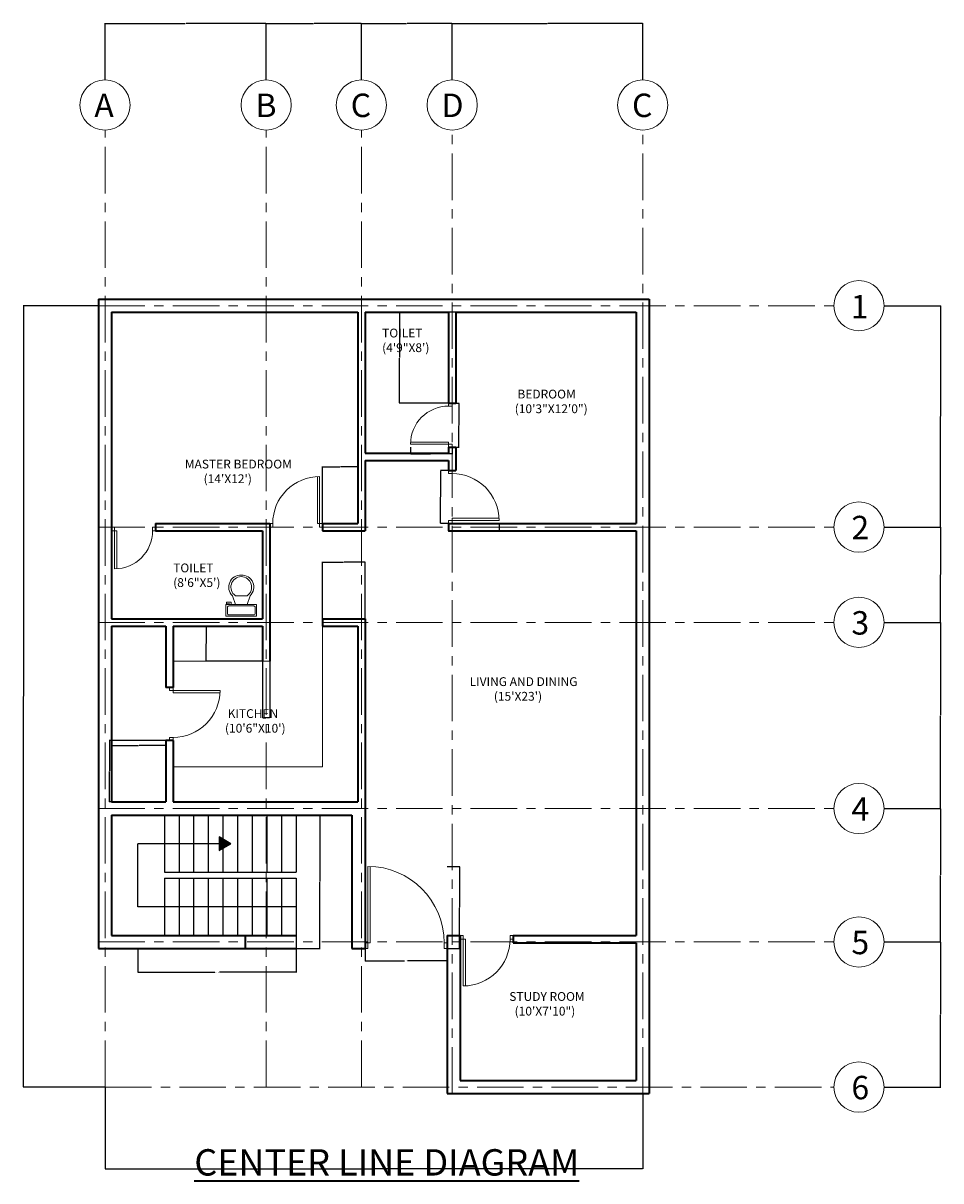
# Model space of a CAD drawing. Units: inches. Extents: x 2948 to 4025, y 2171 to 2966.
# Tile 6 of 6: x 3398 to 4025, y 2177 to 2966. Entities that reach past the tile are written whole.
import ezdxf

# ---------------------------------------------------------------- set-up
doc = ezdxf.new("R2010")
doc.units = ezdxf.units.IN
doc.linetypes.add('CENTER', pattern=[50.8, 31.75, -6.35, 6.35, -6.35])
for name, color, linetype, lineweight in [('A-ANNO-DIMS', 2, 'Continuous', 18), ('A-ANNO-TEXT', 7, 'Continuous', 35), ('A-AREA-IDEN', 7, 'Continuous', 18), ('A-DOOR', 3, 'Continuous', 18), ('A-FLOR-CASE', 8, 'Continuous', 18), ('A-FLOR-FIXT', 9, 'Continuous', 18), ('A-FLOR-STRS', 7, 'Continuous', 25), ('A-GRID', 1, 'CENTER', 13), ('A-GRID-IDEN', 7, 'Continuous', 18), ('A-WALL', 7, 'Continuous', 35)]:
    doc.layers.add(name, color=color, linetype=linetype, lineweight=lineweight)
doc.styles.get("Standard").update_dxf_attribs({"font": 'arial.ttf'})
doc.dimstyles.get("Standard").update_dxf_attribs({"dimtxt": 0.18, "dimasz": 0.18, "dimexe": 0.18, "dimexo": 0.0625, "dimgap": 0.09, "dimtad": 0, "dimtih": 1, "dimtoh": 1, "dimdec": 4, "dimzin": 0, "dimdsep": 46, "dimtxsty": 'Standard', "dimcen": 0.09, "dimadec": 0, "dimazin": 0, "dimtfac": 1, "dimtdec": 4, "dimtofl": 0, "dimtmove": 0, "dimatfit": 3, "dimfxl": 1, "dimtolj": 1, "dimtzin": 0, "dimarcsym": 0})

# ---------------------------------------------------------------- blocks, each defined once
blk = doc.blocks.new('*U8')
for p, q in [((9.5, -6), (9.5, -2)), ((-10, -8.5), (-8, -8.5)), ((-10, -9.5), (-10, -8.5)), ((-7, -9.5), (-10, -9.5)), ((-8, -8.5), (-8, -8)), ((-7, -8), (-7, -9.5)), ((-4, -8), (-6, -14)), ((4, -14), (-4, -14)), ((4, -8), (6, -14))]:
    blk.add_line(p, q)
blk.add_lwpolyline([(10.5, -8), (10.5, 0), (-10.5, 0), (-10.5, -8)], close=True)
for points in [[(-9.5, -2), (-9.5, -6)], [(8.5, -1), (-8.5, -1)], [(-8.5, -7), (8.5, -7)]]:
    blk.add_lwpolyline(points)
for centre, radius, start, end in [((-8.625, -1.875), 0.8839, 81.8699, 188.1301), ((-8.625, -6.125), 0.8839, 171.869898, 278.1301), ((8.625, -1.875), 0.8839, 351.8699, 98.1301), ((8.625, -6.125), 0.8839, 261.8699, 8.1301), ((-0.4772, -19.9188), 8.0953, 133.01722, 273.38), ((0.0374, -19.8731), 7.127, 124.50543, 269.7), ((-0.0373, -19.8731), 7.127, 270.3, 55.4946), ((0.4773, -19.9188), 8.0953, 266.62, 46.9828)]:
    blk.add_arc(centre, radius, start, end)
blk = doc.blocks.new('DOOR-SWING-32IN')
for p, q in [((2, 34.5), (0, 34.5)), ((0, 32), (2, 32)), ((2, 32), (2, 34.5)), ((2, 32), (2, 0)), ((2, 32), (3.5, 32)), ((3.5, 32), (3.5, 0.04)), ((34, 32), (34, 34.5)), ((34, 34.5), (36, 34.5)), ((36, 32), (34, 32))]:
    blk.add_line(p, q)
blk.add_arc((2, 32), 32, 270, 0)
blk = doc.blocks.new('DOOR-SWING-26IN')
for p, q in [((26, 30), (26, 28)), ((26, 28), (28.5, 28)), ((28.5, 28), (28.5, 30)), ((26, 2), (0, 2)), ((26, 3.5), (0.04, 3.5)), ((26, 3.5), (26, 2)), ((26, 0), (26, 2)), ((26, 2), (28.5, 2)), ((28.5, 2), (28.5, 0))]:
    blk.add_line(p, q)
blk.add_arc((26, 2), 26, 90, 180)
blk = doc.blocks.new('DOOR-ENTRY-52IN')
for p, q in [((2, 4), (2, 56)), ((3.5, 4), (3.5, 55.98)), ((2, 4), (0, 4)), ((0, 0), (2, 0)), ((2, 0), (2, 4)), ((2, 4), (3.5, 4)), ((54, 0), (54, 4)), ((54, 4), (56, 4)), ((56, 0), (54, 0))]:
    blk.add_line(p, q)
blk.add_arc((2, 4), 52, 0, 90)
blk = doc.blocks.new('STAIR-RETURN-FLIGHT')
h = blk.add_hatch(color=256)
h.dxf.hatch_style = 1
h.paths.add_polyline_path([(63.35, 71.5), (55.35, 76.12), (55.35, 66.88)])
for p, q in [((18.02, 91), (18.02, 52)), ((28.02, 91), (28.02, 52)), ((38.02, 91), (38.02, 52)), ((48.02, 91), (48.02, 52)), ((58.02, 91), (58.02, 74.58)), ((68.02, 91), (68.02, 52)), ((78.02, 91), (78.02, 52)), ((88.02, 91), (88.02, 52)), ((98.02, 91), (98.02, 52)), ((108.02, 91), (108.02, 52)), ((0, 28.5), (0, 71.5)), ((55.35, 71.5), (0, 71.5)), ((58.02, 68.42), (58.02, 52)), ((18.02, 52), (108.02, 52)), ((18.02, 48), (108.02, 48)), ((18.02, 48), (18.02, 9)), ((28.02, 48), (28.02, 9)), ((38.02, 48), (38.02, 9)), ((48.02, 48), (48.02, 9)), ((58.02, 48), (58.02, 9)), ((68.02, 48), (68.02, 9)), ((78.02, 48), (78.02, 9)), ((88.02, 48), (88.02, 9)), ((98.02, 48), (98.02, 9)), ((108.02, 48), (108.02, 0)), ((108.02, 28.5), (0, 28.5))]:
    blk.add_line(p, q)
blk.add_lwpolyline([(63.35, 71.5), (55.35, 76.12), (55.35, 66.88)], close=True)
blk = doc.blocks.new('*D15')
at = {"layer": 'A-ANNO-DIMS', "color": 0, "lineweight": -2, "transparency": 16777216}
for p, q in [((3688.78, 2660.99), (3683.26, 2660.99)), ((3683.44, 2660.81), (3683.44, 2643.17)), ((3683.44, 2625.17), (3683.44, 2642.8)), ((3688.78, 2624.99), (3683.26, 2624.99))]:
    blk.add_line(p, q, dxfattribs=at)
at = {"layer": 'A-ANNO-DIMS', "color": 0, "transparency": 16777216}
for points in [[(3683.41, 2660.81), (3683.47, 2660.81), (3683.44, 2660.99)], [(3683.41, 2625.17), (3683.47, 2625.17), (3683.44, 2624.99)]]:
    blk.add_solid(points, dxfattribs=at)
at = {"layer": 'Defpoints', "color": 0, "transparency": 16777216}
for p in [(3683.44, 2660.99), (3688.84, 2660.99), (3688.84, 2624.99)]:
    blk.add_point(p, dxfattribs=at)
at = {"layer": 'A-ANNO-DIMS', "color": 0, "transparency": 16777216, "insert": (3683.44, 2642.99), "char_height": 0.18, "attachment_point": 5}
blk.add_mtext('\\A1;ROOM DOOR 36 TYP.', dxfattribs=at)
blk = doc.blocks.new('*D16')
at = {"layer": 'A-ANNO-DIMS', "color": 0, "lineweight": -2, "transparency": 16777216}
for p, q in [((3688.84, 2624.92), (3688.84, 2619.41)), ((3723.34, 2624.92), (3723.34, 2619.41)), ((3689.02, 2619.59), (3705.56, 2619.59)), ((3723.16, 2619.59), (3706.62, 2619.59))]:
    blk.add_line(p, q, dxfattribs=at)
at = {"layer": 'A-ANNO-DIMS', "color": 0, "transparency": 16777216}
for points in [[(3689.02, 2619.62), (3689.02, 2619.56), (3688.84, 2619.59)], [(3723.16, 2619.62), (3723.16, 2619.56), (3723.34, 2619.59)]]:
    blk.add_solid(points, dxfattribs=at)
at = {"layer": 'Defpoints', "color": 0, "transparency": 16777216}
for p in [(3688.84, 2624.99), (3723.34, 2624.99), (3688.84, 2619.59)]:
    blk.add_point(p, dxfattribs=at)
at = {"layer": 'A-ANNO-DIMS', "color": 0, "transparency": 16777216, "insert": (3706.09, 2619.59), "char_height": 0.18, "attachment_point": 5}
blk.add_mtext('\\A1;35 TYP.', dxfattribs=at)
blk = doc.blocks.new('*D17')
at = {"layer": 'A-ANNO-DIMS', "color": 0, "lineweight": -2, "transparency": 16777216}
for p, q in [((3691.4, 2706.99), (3696.02, 2706.99)), ((3695.84, 2706.81), (3695.84, 2692.17)), ((3695.84, 2677.17), (3695.84, 2691.8)), ((3691.4, 2676.99), (3696.02, 2676.99))]:
    blk.add_line(p, q, dxfattribs=at)
at = {"layer": 'A-ANNO-DIMS', "color": 0, "transparency": 16777216}
for points in [[(3695.81, 2706.81), (3695.87, 2706.81), (3695.84, 2706.99)], [(3695.81, 2677.17), (3695.87, 2677.17), (3695.84, 2676.99)]]:
    blk.add_solid(points, dxfattribs=at)
at = {"layer": 'Defpoints', "color": 0, "transparency": 16777216}
for p in [(3691.34, 2706.99), (3695.84, 2706.99), (3691.34, 2676.99)]:
    blk.add_point(p, dxfattribs=at)
at = {"layer": 'A-ANNO-DIMS', "color": 0, "transparency": 16777216, "insert": (3695.84, 2691.99), "char_height": 0.18, "attachment_point": 5}
blk.add_mtext('\\A1;WC DOOR 30 TYP.', dxfattribs=at)
blk = doc.blocks.new('*D18')
at = {"layer": 'A-ANNO-DIMS', "color": 0, "lineweight": -2, "transparency": 16777216}
for p, q in [((3662.84, 2676.92), (3662.84, 2672.31)), ((3663.02, 2672.49), (3676.56, 2672.49)), ((3691.16, 2672.49), (3677.62, 2672.49)), ((3691.34, 2676.92), (3691.34, 2672.31))]:
    blk.add_line(p, q, dxfattribs=at)
at = {"layer": 'A-ANNO-DIMS', "color": 0, "transparency": 16777216}
for points in [[(3663.02, 2672.52), (3663.02, 2672.46), (3662.84, 2672.49)], [(3691.16, 2672.52), (3691.16, 2672.46), (3691.34, 2672.49)]]:
    blk.add_solid(points, dxfattribs=at)
at = {"layer": 'Defpoints', "color": 0, "transparency": 16777216}
for p in [(3662.84, 2676.99), (3691.34, 2676.99), (3691.34, 2672.49)]:
    blk.add_point(p, dxfattribs=at)
at = {"layer": 'A-ANNO-DIMS', "color": 0, "transparency": 16777216, "insert": (3677.09, 2672.49), "char_height": 0.18, "attachment_point": 5}
blk.add_mtext('\\A1;29 TYP.', dxfattribs=at)
blk = doc.blocks.new('*D19')
at = {"layer": 'A-ANNO-DIMS', "color": 0, "lineweight": -2, "transparency": 16777216}
for p, q in [((3631.84, 2334.92), (3631.84, 2326.41)), ((3687.84, 2334.92), (3687.84, 2326.41)), ((3632.02, 2326.59), (3658.85, 2326.59)), ((3687.66, 2326.59), (3660.82, 2326.59))]:
    blk.add_line(p, q, dxfattribs=at)
at = {"layer": 'A-ANNO-DIMS', "color": 0, "transparency": 16777216}
for points in [[(3632.02, 2326.62), (3632.02, 2326.56), (3631.84, 2326.59)], [(3687.66, 2326.62), (3687.66, 2326.56), (3687.84, 2326.59)]]:
    blk.add_solid(points, dxfattribs=at)
at = {"layer": 'Defpoints', "color": 0, "transparency": 16777216}
for p in [(3631.84, 2334.99), (3687.84, 2334.99), (3687.84, 2326.59)]:
    blk.add_point(p, dxfattribs=at)
at = {"layer": 'A-ANNO-DIMS', "color": 0, "transparency": 16777216, "insert": (3659.84, 2326.59), "char_height": 0.18, "attachment_point": 5}
blk.add_mtext('\\A1;ENTRY 56 TYP.', dxfattribs=at)
blk = doc.blocks.new('*D20')
at = {"layer": 'A-ANNO-DIMS', "color": 0, "lineweight": -2, "transparency": 16777216}
for p, q in [((3687.9, 2390.99), (3696.42, 2390.99)), ((3696.24, 2390.81), (3696.24, 2363.17)), ((3696.24, 2335.17), (3696.24, 2362.8)), ((3687.9, 2334.99), (3696.42, 2334.99))]:
    blk.add_line(p, q, dxfattribs=at)
at = {"layer": 'A-ANNO-DIMS', "color": 0, "transparency": 16777216}
for points in [[(3696.21, 2390.81), (3696.27, 2390.81), (3696.24, 2390.99)], [(3696.21, 2335.17), (3696.27, 2335.17), (3696.24, 2334.99)]]:
    blk.add_solid(points, dxfattribs=at)
at = {"layer": 'Defpoints', "color": 0, "transparency": 16777216}
for p in [(3687.84, 2390.99), (3696.24, 2390.99), (3687.84, 2334.99)]:
    blk.add_point(p, dxfattribs=at)
at = {"layer": 'A-ANNO-DIMS', "color": 0, "transparency": 16777216, "insert": (3696.24, 2362.99), "char_height": 0.18, "attachment_point": 5}
blk.add_mtext('\\A1;56 TYP.', dxfattribs=at)
blk = doc.blocks.new('*D25')
at = {"layer": 'A-ANNO-DIMS', "color": 0, "lineweight": -2, "transparency": 16777216}
for p, q in [((3476.82, 2334.92), (3476.82, 2318.6)), ((3584.84, 2334.92), (3584.84, 2318.6)), ((3477, 2318.78), (3529.27, 2318.78)), ((3584.66, 2318.78), (3532.39, 2318.78))]:
    blk.add_line(p, q, dxfattribs=at)
at = {"layer": 'A-ANNO-DIMS', "color": 0, "transparency": 16777216}
for points in [[(3477, 2318.81), (3477, 2318.75), (3476.82, 2318.78)], [(3584.66, 2318.81), (3584.66, 2318.75), (3584.84, 2318.78)]]:
    blk.add_solid(points, dxfattribs=at)
at = {"layer": 'Defpoints', "color": 0, "transparency": 16777216}
for p in [(3476.82, 2334.99), (3584.84, 2334.99), (3584.84, 2318.78)]:
    blk.add_point(p, dxfattribs=at)
at = {"layer": 'A-ANNO-DIMS', "color": 0, "transparency": 16777216, "insert": (3530.83, 2318.78), "char_height": 0.18, "attachment_point": 5}
blk.add_mtext('\\A1;RETURN STAIR 108 TYP.', dxfattribs=at)
blk = doc.blocks.new('*D26')
at = {"layer": 'A-ANNO-DIMS', "color": 0, "lineweight": -2, "transparency": 16777216}
for p, q in [((3584.9, 2425.99), (3601.22, 2425.99)), ((3601.04, 2425.81), (3601.04, 2380.67)), ((3601.04, 2335.17), (3601.04, 2380.3)), ((3584.9, 2334.99), (3601.22, 2334.99))]:
    blk.add_line(p, q, dxfattribs=at)
at = {"layer": 'A-ANNO-DIMS', "color": 0, "transparency": 16777216}
for points in [[(3601.01, 2425.81), (3601.07, 2425.81), (3601.04, 2425.99)], [(3601.01, 2335.17), (3601.07, 2335.17), (3601.04, 2334.99)]]:
    blk.add_solid(points, dxfattribs=at)
at = {"layer": 'Defpoints', "color": 0, "transparency": 16777216}
for p in [(3584.84, 2425.99), (3601.04, 2425.99), (3584.84, 2334.99)]:
    blk.add_point(p, dxfattribs=at)
at = {"layer": 'A-ANNO-DIMS', "color": 0, "transparency": 16777216, "insert": (3601.04, 2380.49), "char_height": 0.18, "attachment_point": 5}
blk.add_mtext('\\A1;91 TYP.', dxfattribs=at)
blk = doc.blocks.new('*D49')
at = {"layer": 'A-ANNO-DIMS', "color": 0, "lineweight": -2, "transparency": 16777216}
for p, q in [((3454.34, 2927.56), (3454.34, 2966.23)), ((3454.52, 2966.05), (3509.06, 2966.05)), ((3564.16, 2966.05), (3509.62, 2966.05)), ((3564.34, 2927.56), (3564.34, 2966.23))]:
    blk.add_line(p, q, dxfattribs=at)
at = {"layer": 'A-ANNO-DIMS', "color": 0, "transparency": 16777216}
for points in [[(3454.52, 2966.08), (3454.52, 2966.02), (3454.34, 2966.05)], [(3564.16, 2966.08), (3564.16, 2966.02), (3564.34, 2966.05)]]:
    blk.add_solid(points, dxfattribs=at)
at = {"layer": 'Defpoints', "color": 0, "transparency": 16777216}
for p in [(3564.34, 2966.05), (3454.34, 2927.5), (3564.34, 2927.5)]:
    blk.add_point(p, dxfattribs=at)
at = {"layer": 'A-ANNO-DIMS', "color": 0, "transparency": 16777216, "insert": (3509.34, 2966.05), "char_height": 0.18, "attachment_point": 5}
blk.add_mtext('\\A1;110', dxfattribs=at)
blk = doc.blocks.new('*D50')
at = {"layer": 'A-ANNO-DIMS', "color": 0, "lineweight": -2, "transparency": 16777216}
for p, q in [((3564.34, 2927.56), (3564.34, 2966.23)), ((3564.52, 2966.05), (3596.62, 2966.05)), ((3629.16, 2966.05), (3597.06, 2966.05)), ((3629.34, 2927.56), (3629.34, 2966.23))]:
    blk.add_line(p, q, dxfattribs=at)
at = {"layer": 'A-ANNO-DIMS', "color": 0, "transparency": 16777216}
for points in [[(3564.52, 2966.08), (3564.52, 2966.02), (3564.34, 2966.05)], [(3629.16, 2966.08), (3629.16, 2966.02), (3629.34, 2966.05)]]:
    blk.add_solid(points, dxfattribs=at)
at = {"layer": 'Defpoints', "color": 0, "transparency": 16777216}
for p in [(3629.34, 2966.05), (3564.34, 2927.5), (3629.34, 2927.5)]:
    blk.add_point(p, dxfattribs=at)
at = {"layer": 'A-ANNO-DIMS', "color": 0, "transparency": 16777216, "insert": (3596.84, 2966.05), "char_height": 0.18, "attachment_point": 5}
blk.add_mtext('\\A1;65', dxfattribs=at)
blk = doc.blocks.new('*D51')
at = {"layer": 'A-ANNO-DIMS', "color": 0, "lineweight": -2, "transparency": 16777216}
for p, q in [((3629.34, 2927.56), (3629.34, 2966.23)), ((3629.52, 2966.05), (3660.12, 2966.05)), ((3691.16, 2966.05), (3660.56, 2966.05)), ((3691.34, 2927.56), (3691.34, 2966.23))]:
    blk.add_line(p, q, dxfattribs=at)
at = {"layer": 'A-ANNO-DIMS', "color": 0, "transparency": 16777216}
for points in [[(3629.52, 2966.08), (3629.52, 2966.02), (3629.34, 2966.05)], [(3691.16, 2966.08), (3691.16, 2966.02), (3691.34, 2966.05)]]:
    blk.add_solid(points, dxfattribs=at)
at = {"layer": 'Defpoints', "color": 0, "transparency": 16777216}
for p in [(3691.34, 2966.05), (3629.34, 2927.5), (3691.34, 2927.5)]:
    blk.add_point(p, dxfattribs=at)
at = {"layer": 'A-ANNO-DIMS', "color": 0, "transparency": 16777216, "insert": (3660.34, 2966.05), "char_height": 0.18, "attachment_point": 5}
blk.add_mtext('\\A1;62', dxfattribs=at)
blk = doc.blocks.new('*D52')
at = {"layer": 'A-ANNO-DIMS', "color": 0, "lineweight": -2, "transparency": 16777216}
for p, q in [((3691.34, 2927.56), (3691.34, 2966.23)), ((3691.52, 2966.05), (3756.06, 2966.05)), ((3821.16, 2966.05), (3756.62, 2966.05)), ((3821.34, 2927.56), (3821.34, 2966.23))]:
    blk.add_line(p, q, dxfattribs=at)
at = {"layer": 'A-ANNO-DIMS', "color": 0, "transparency": 16777216}
for points in [[(3691.52, 2966.08), (3691.52, 2966.02), (3691.34, 2966.05)], [(3821.16, 2966.08), (3821.16, 2966.02), (3821.34, 2966.05)]]:
    blk.add_solid(points, dxfattribs=at)
at = {"layer": 'Defpoints', "color": 0, "transparency": 16777216}
for p in [(3821.34, 2966.05), (3691.34, 2927.5), (3821.34, 2927.5)]:
    blk.add_point(p, dxfattribs=at)
at = {"layer": 'A-ANNO-DIMS', "color": 0, "transparency": 16777216, "insert": (3756.34, 2966.05), "char_height": 0.18, "attachment_point": 5}
blk.add_mtext('\\A1;130', dxfattribs=at)
blk = doc.blocks.new('*D53')
at = {"layer": 'A-ANNO-DIMS', "color": 0, "lineweight": -2, "transparency": 16777216}
for p, q in [((3454.34, 2240.42), (3454.34, 2184.63)), ((3821.34, 2235.92), (3821.34, 2184.63)), ((3454.52, 2184.81), (3637.55, 2184.81)), ((3821.16, 2184.81), (3638.13, 2184.81))]:
    blk.add_line(p, q, dxfattribs=at)
at = {"layer": 'A-ANNO-DIMS', "color": 0, "transparency": 16777216}
for points in [[(3454.52, 2184.84), (3454.52, 2184.78), (3454.34, 2184.81)], [(3821.16, 2184.84), (3821.16, 2184.78), (3821.34, 2184.81)]]:
    blk.add_solid(points, dxfattribs=at)
at = {"layer": 'Defpoints', "color": 0, "transparency": 16777216}
for p in [(3454.34, 2240.49), (3821.34, 2235.99), (3821.34, 2184.81)]:
    blk.add_point(p, dxfattribs=at)
at = {"layer": 'A-ANNO-DIMS', "color": 0, "transparency": 16777216, "insert": (3637.84, 2184.81), "char_height": 0.18, "attachment_point": 5}
blk.add_mtext('\\A1;367', dxfattribs=at)
blk = doc.blocks.new('*D54')
at = {"layer": 'A-ANNO-DIMS', "color": 0, "lineweight": -2, "transparency": 16777216}
for p, q in [((3986.17, 2773.49), (4024.84, 2773.49)), ((4024.66, 2773.31), (4024.66, 2698.17)), ((4024.66, 2622.67), (4024.66, 2697.8)), ((3986.17, 2622.49), (4024.84, 2622.49))]:
    blk.add_line(p, q, dxfattribs=at)
at = {"layer": 'A-ANNO-DIMS', "color": 0, "transparency": 16777216}
for points in [[(4024.63, 2773.31), (4024.69, 2773.31), (4024.66, 2773.49)], [(4024.63, 2622.67), (4024.69, 2622.67), (4024.66, 2622.49)]]:
    blk.add_solid(points, dxfattribs=at)
at = {"layer": 'Defpoints', "color": 0, "transparency": 16777216}
for p in [(3986.11, 2773.49), (4024.66, 2773.49), (3986.11, 2622.49)]:
    blk.add_point(p, dxfattribs=at)
at = {"layer": 'A-ANNO-DIMS', "color": 0, "transparency": 16777216, "insert": (4024.66, 2697.99), "char_height": 0.18, "attachment_point": 5}
blk.add_mtext('\\A1;151', dxfattribs=at)
blk = doc.blocks.new('*D55')
at = {"layer": 'A-ANNO-DIMS', "color": 0, "lineweight": -2, "transparency": 16777216}
for p, q in [((3986.17, 2622.49), (4024.84, 2622.49)), ((4024.66, 2622.31), (4024.66, 2590.17)), ((4024.66, 2557.67), (4024.66, 2589.8)), ((3986.17, 2557.49), (4024.84, 2557.49))]:
    blk.add_line(p, q, dxfattribs=at)
at = {"layer": 'A-ANNO-DIMS', "color": 0, "transparency": 16777216}
for points in [[(4024.63, 2622.31), (4024.69, 2622.31), (4024.66, 2622.49)], [(4024.63, 2557.67), (4024.69, 2557.67), (4024.66, 2557.49)]]:
    blk.add_solid(points, dxfattribs=at)
at = {"layer": 'Defpoints', "color": 0, "transparency": 16777216}
for p in [(3986.11, 2622.49), (4024.66, 2622.49), (3986.11, 2557.49)]:
    blk.add_point(p, dxfattribs=at)
at = {"layer": 'A-ANNO-DIMS', "color": 0, "transparency": 16777216, "insert": (4024.66, 2589.99), "char_height": 0.18, "attachment_point": 5}
blk.add_mtext('\\A1;65', dxfattribs=at)
blk = doc.blocks.new('*D56')
at = {"layer": 'A-ANNO-DIMS', "color": 0, "lineweight": -2, "transparency": 16777216}
for p, q in [((3986.17, 2557.49), (4024.84, 2557.49)), ((4024.66, 2557.31), (4024.66, 2494.17)), ((4024.66, 2430.67), (4024.66, 2493.81)), ((3986.17, 2430.49), (4024.84, 2430.49))]:
    blk.add_line(p, q, dxfattribs=at)
at = {"layer": 'A-ANNO-DIMS', "color": 0, "transparency": 16777216}
for points in [[(4024.63, 2557.31), (4024.69, 2557.31), (4024.66, 2557.49)], [(4024.63, 2430.67), (4024.69, 2430.67), (4024.66, 2430.49)]]:
    blk.add_solid(points, dxfattribs=at)
at = {"layer": 'Defpoints', "color": 0, "transparency": 16777216}
for p in [(3986.11, 2557.49), (4024.66, 2557.49), (3986.11, 2430.49)]:
    blk.add_point(p, dxfattribs=at)
at = {"layer": 'A-ANNO-DIMS', "color": 0, "transparency": 16777216, "insert": (4024.66, 2493.99), "char_height": 0.18, "attachment_point": 5}
blk.add_mtext('\\A1;127', dxfattribs=at)
blk = doc.blocks.new('*D57')
at = {"layer": 'A-ANNO-DIMS', "color": 0, "lineweight": -2, "transparency": 16777216}
for p, q in [((3986.17, 2430.49), (4024.84, 2430.49)), ((4024.66, 2430.31), (4024.66, 2385.17)), ((4024.66, 2339.67), (4024.66, 2384.8)), ((3986.17, 2339.49), (4024.84, 2339.49))]:
    blk.add_line(p, q, dxfattribs=at)
at = {"layer": 'A-ANNO-DIMS', "color": 0, "transparency": 16777216}
for points in [[(4024.63, 2430.31), (4024.69, 2430.31), (4024.66, 2430.49)], [(4024.63, 2339.67), (4024.69, 2339.67), (4024.66, 2339.49)]]:
    blk.add_solid(points, dxfattribs=at)
at = {"layer": 'Defpoints', "color": 0, "transparency": 16777216}
for p in [(3986.11, 2430.49), (4024.66, 2430.49), (3986.11, 2339.49)]:
    blk.add_point(p, dxfattribs=at)
at = {"layer": 'A-ANNO-DIMS', "color": 0, "transparency": 16777216, "insert": (4024.66, 2384.99), "char_height": 0.18, "attachment_point": 5}
blk.add_mtext('\\A1;91', dxfattribs=at)
blk = doc.blocks.new('*D58')
at = {"layer": 'A-ANNO-DIMS', "color": 0, "lineweight": -2, "transparency": 16777216}
for p, q in [((3986.17, 2339.49), (4024.84, 2339.49)), ((4024.66, 2339.31), (4024.66, 2290.17)), ((4024.66, 2240.67), (4024.66, 2289.8)), ((3986.17, 2240.49), (4024.84, 2240.49))]:
    blk.add_line(p, q, dxfattribs=at)
at = {"layer": 'A-ANNO-DIMS', "color": 0, "transparency": 16777216}
for points in [[(4024.63, 2339.31), (4024.69, 2339.31), (4024.66, 2339.49)], [(4024.63, 2240.67), (4024.69, 2240.67), (4024.66, 2240.49)]]:
    blk.add_solid(points, dxfattribs=at)
at = {"layer": 'Defpoints', "color": 0, "transparency": 16777216}
for p in [(3986.11, 2339.49), (4024.66, 2339.49), (3986.11, 2240.49)]:
    blk.add_point(p, dxfattribs=at)
at = {"layer": 'A-ANNO-DIMS', "color": 0, "transparency": 16777216, "insert": (4024.66, 2289.99), "char_height": 0.18, "attachment_point": 5}
blk.add_mtext('\\A1;99', dxfattribs=at)
blk = doc.blocks.new('*D59')
at = {"layer": 'A-ANNO-DIMS', "color": 0, "lineweight": -2, "transparency": 16777216}
for p, q in [((3449.78, 2773.49), (3398.48, 2773.49)), ((3398.66, 2773.31), (3398.66, 2507.17)), ((3398.66, 2240.67), (3398.66, 2506.8)), ((3454.28, 2240.49), (3398.48, 2240.49))]:
    blk.add_line(p, q, dxfattribs=at)
at = {"layer": 'A-ANNO-DIMS', "color": 0, "transparency": 16777216}
for points in [[(3398.63, 2773.31), (3398.69, 2773.31), (3398.66, 2773.49)], [(3398.63, 2240.67), (3398.69, 2240.67), (3398.66, 2240.49)]]:
    blk.add_solid(points, dxfattribs=at)
at = {"layer": 'Defpoints', "color": 0, "transparency": 16777216}
for p in [(3398.66, 2773.49), (3449.84, 2773.49), (3454.34, 2240.49)]:
    blk.add_point(p, dxfattribs=at)
at = {"layer": 'A-ANNO-DIMS', "color": 0, "transparency": 16777216, "insert": (3398.66, 2506.99), "char_height": 0.18, "attachment_point": 5}
blk.add_mtext('\\A1;533', dxfattribs=at)
blk = doc.blocks.new('*D60')
at = {"layer": 'A-ANNO-DIMS', "color": 0, "lineweight": -2, "transparency": 16777216}
for p, q in [((3458.84, 2435.05), (3458.84, 2473.72)), ((3459.02, 2473.54), (3477.12, 2473.54)), ((3495.66, 2473.54), (3477.56, 2473.54)), ((3495.84, 2435.05), (3495.84, 2473.72))]:
    blk.add_line(p, q, dxfattribs=at)
at = {"layer": 'A-ANNO-DIMS', "color": 0, "transparency": 16777216}
for points in [[(3459.02, 2473.57), (3459.02, 2473.51), (3458.84, 2473.54)], [(3495.66, 2473.57), (3495.66, 2473.51), (3495.84, 2473.54)]]:
    blk.add_solid(points, dxfattribs=at)
at = {"layer": 'Defpoints', "color": 0, "transparency": 16777216}
for p in [(3495.84, 2473.54), (3458.84, 2434.99), (3495.84, 2434.99)]:
    blk.add_point(p, dxfattribs=at)
at = {"layer": 'A-ANNO-DIMS', "color": 0, "transparency": 16777216, "insert": (3477.34, 2473.54), "char_height": 0.18, "attachment_point": 5}
blk.add_mtext('\\A1;37', dxfattribs=at)
blk = doc.blocks.new('*D61')
at = {"layer": 'A-ANNO-DIMS', "color": 0, "lineweight": -2, "transparency": 16777216}
for p, q in [((3495.78, 2476.99), (3457.11, 2476.99)), ((3457.29, 2476.81), (3457.29, 2456.17)), ((3457.29, 2435.17), (3457.29, 2455.81)), ((3495.78, 2434.99), (3457.11, 2434.99))]:
    blk.add_line(p, q, dxfattribs=at)
at = {"layer": 'A-ANNO-DIMS', "color": 0, "transparency": 16777216}
for points in [[(3457.26, 2476.81), (3457.32, 2476.81), (3457.29, 2476.99)], [(3457.26, 2435.17), (3457.32, 2435.17), (3457.29, 2434.99)]]:
    blk.add_solid(points, dxfattribs=at)
at = {"layer": 'Defpoints', "color": 0, "transparency": 16777216}
for p in [(3457.29, 2476.99), (3495.84, 2476.99), (3495.84, 2434.99)]:
    blk.add_point(p, dxfattribs=at)
at = {"layer": 'A-ANNO-DIMS', "color": 0, "transparency": 16777216, "insert": (3457.29, 2455.99), "char_height": 0.18, "attachment_point": 5}
blk.add_mtext('\\A1;42', dxfattribs=at)
blk = doc.blocks.new('*D62')
at = {"layer": 'A-ANNO-DIMS', "color": 0, "lineweight": -2, "transparency": 16777216}
for p, q in [((3561.78, 2554.99), (3523.11, 2554.99)), ((3523.29, 2554.81), (3523.29, 2543.17)), ((3523.29, 2531.17), (3523.29, 2542.81)), ((3561.78, 2530.99), (3523.11, 2530.99))]:
    blk.add_line(p, q, dxfattribs=at)
at = {"layer": 'A-ANNO-DIMS', "color": 0, "transparency": 16777216}
for points in [[(3523.26, 2554.81), (3523.32, 2554.81), (3523.29, 2554.99)], [(3523.26, 2531.17), (3523.32, 2531.17), (3523.29, 2530.99)]]:
    blk.add_solid(points, dxfattribs=at)
at = {"layer": 'Defpoints', "color": 0, "transparency": 16777216}
for p in [(3523.29, 2554.99), (3561.84, 2554.99), (3561.84, 2530.99)]:
    blk.add_point(p, dxfattribs=at)
at = {"layer": 'A-ANNO-DIMS', "color": 0, "transparency": 16777216, "insert": (3523.29, 2542.99), "char_height": 0.18, "attachment_point": 5}
blk.add_mtext('\\A1;24', dxfattribs=at)
blk = doc.blocks.new('*D63')
at = {"layer": 'A-ANNO-DIMS', "color": 0, "lineweight": -2, "transparency": 16777216}
for p, q in [((3602.84, 2560.05), (3602.84, 2598.72)), ((3603.02, 2598.54), (3617.12, 2598.54)), ((3631.66, 2598.54), (3617.56, 2598.54)), ((3631.84, 2560.05), (3631.84, 2598.72))]:
    blk.add_line(p, q, dxfattribs=at)
at = {"layer": 'A-ANNO-DIMS', "color": 0, "transparency": 16777216}
for points in [[(3603.02, 2598.57), (3603.02, 2598.51), (3602.84, 2598.54)], [(3631.66, 2598.57), (3631.66, 2598.51), (3631.84, 2598.54)]]:
    blk.add_solid(points, dxfattribs=at)
at = {"layer": 'Defpoints', "color": 0, "transparency": 16777216}
for p in [(3631.84, 2598.54), (3602.84, 2559.99), (3631.84, 2559.99)]:
    blk.add_point(p, dxfattribs=at)
at = {"layer": 'A-ANNO-DIMS', "color": 0, "transparency": 16777216, "insert": (3617.34, 2598.54), "char_height": 0.18, "attachment_point": 5}
blk.add_mtext('\\A1;29', dxfattribs=at)
blk = doc.blocks.new('*D64')
at = {"layer": 'A-ANNO-DIMS', "color": 0, "lineweight": -2, "transparency": 16777216}
for p, q in [((3602.84, 2625.05), (3602.84, 2663.72)), ((3603.02, 2663.54), (3614.62, 2663.54)), ((3626.66, 2663.54), (3615.06, 2663.54)), ((3626.84, 2625.05), (3626.84, 2663.72))]:
    blk.add_line(p, q, dxfattribs=at)
at = {"layer": 'A-ANNO-DIMS', "color": 0, "transparency": 16777216}
for points in [[(3603.02, 2663.57), (3603.02, 2663.51), (3602.84, 2663.54)], [(3626.66, 2663.57), (3626.66, 2663.51), (3626.84, 2663.54)]]:
    blk.add_solid(points, dxfattribs=at)
at = {"layer": 'Defpoints', "color": 0, "transparency": 16777216}
for p in [(3626.84, 2663.54), (3602.84, 2624.99), (3626.84, 2624.99)]:
    blk.add_point(p, dxfattribs=at)
at = {"layer": 'A-ANNO-DIMS', "color": 0, "transparency": 16777216, "insert": (3614.84, 2663.54), "char_height": 0.18, "attachment_point": 5}
blk.add_mtext('\\A1;24', dxfattribs=at)
blk = doc.blocks.new('*D65')
at = {"layer": 'A-ANNO-DIMS', "color": 0, "lineweight": -2, "transparency": 16777216}
for p, q in [((3561.84, 2530.92), (3561.84, 2492.26)), ((3566.84, 2530.92), (3566.84, 2492.26)), ((3562.02, 2492.44), (3564.19, 2492.44)), ((3566.66, 2492.44), (3564.49, 2492.44))]:
    blk.add_line(p, q, dxfattribs=at)
at = {"layer": 'A-ANNO-DIMS', "color": 0, "transparency": 16777216}
for points in [[(3562.02, 2492.47), (3562.02, 2492.41), (3561.84, 2492.44)], [(3566.66, 2492.47), (3566.66, 2492.41), (3566.84, 2492.44)]]:
    blk.add_solid(points, dxfattribs=at)
at = {"layer": 'Defpoints', "color": 0, "transparency": 16777216}
for p in [(3561.84, 2530.99), (3566.84, 2530.99), (3561.84, 2492.44)]:
    blk.add_point(p, dxfattribs=at)
at = {"layer": 'A-ANNO-DIMS', "color": 0, "transparency": 16777216, "insert": (3564.34, 2492.44), "char_height": 0.18, "attachment_point": 5}
blk.add_mtext('\\A1;5', dxfattribs=at)
blk = doc.blocks.new('*D66')
at = {"layer": 'A-ANNO-DIMS', "color": 0, "lineweight": -2, "transparency": 16777216}
for p, q in [((3693.78, 2768.99), (3655.11, 2768.99)), ((3655.29, 2768.81), (3655.29, 2738.17)), ((3655.29, 2707.17), (3655.29, 2737.8)), ((3693.78, 2706.99), (3655.11, 2706.99))]:
    blk.add_line(p, q, dxfattribs=at)
at = {"layer": 'A-ANNO-DIMS', "color": 0, "transparency": 16777216}
for points in [[(3655.26, 2768.81), (3655.32, 2768.81), (3655.29, 2768.99)], [(3655.26, 2707.17), (3655.32, 2707.17), (3655.29, 2706.99)]]:
    blk.add_solid(points, dxfattribs=at)
at = {"layer": 'Defpoints', "color": 0, "transparency": 16777216}
for p in [(3655.29, 2768.99), (3693.84, 2768.99), (3693.84, 2706.99)]:
    blk.add_point(p, dxfattribs=at)
at = {"layer": 'A-ANNO-DIMS', "color": 0, "transparency": 16777216, "insert": (3655.29, 2737.99), "char_height": 0.18, "attachment_point": 5}
blk.add_mtext('\\A1;62', dxfattribs=at)

msp = doc.modelspace()

# ---------------------------------------------------------------- linework, layer by layer
at = {"layer": 'A-DOOR'}
msp.add_line((3691.3391, 2626.9862), (3691.3391, 2626.9862), dxfattribs=at)
at = {"layer": 'A-FLOR-CASE'}
for p, q in [((3602.8391, 2559.9862), (3602.8391, 2458.9862)), ((3500.8391, 2530.9862), (3566.8391, 2530.9862)), ((3500.8391, 2458.9862), (3602.8391, 2458.9862))]:
    msp.add_line(p, q, dxfattribs=at)
at = {"layer": 'A-GRID'}
for p, q in [((3454.3391, 2240.4862), (3454.3391, 2893.2413)), ((3564.3391, 2240.4862), (3564.3391, 2893.2413)), ((3629.3391, 2240.4862), (3629.3391, 2893.2413)), ((3691.3391, 2235.9862), (3691.3391, 2893.2413)), ((3821.3391, 2235.9862), (3821.3391, 2893.2413)), ((3449.8391, 2773.4862), (3951.8504, 2773.4862)), ((3449.8391, 2622.4862), (3951.8504, 2622.4862)), ((3449.8391, 2557.4862), (3951.8504, 2557.4862)), ((3449.8391, 2430.4862), (3951.8504, 2430.4862)), ((3449.8391, 2339.4862), (3951.8504, 2339.4862)), ((3454.3391, 2240.4862), (3951.8504, 2240.4862))]:
    msp.add_line(p, q, dxfattribs=at)
at = {"layer": 'A-GRID-IDEN'}
for centre in [(3454.3391, 2910.3701), (3564.3391, 2910.3701), (3629.3391, 2910.3701), (3691.3391, 2910.3701), (3821.3391, 2910.3701), (3968.9791, 2773.4862), (3968.9791, 2622.4862), (3968.9791, 2557.4862), (3968.9791, 2430.4862), (3968.9791, 2339.4862), (3968.9791, 2240.4862)]:
    msp.add_circle(centre, 17.1287, dxfattribs=at)
at = {"layer": 'A-WALL'}
for p, q in [((3449.8391, 2777.9862), (3449.8391, 2334.9862)), ((3449.8391, 2777.9862), (3825.8391, 2777.9862)), ((3825.8391, 2777.9862), (3825.8391, 2235.9862)), ((3458.8391, 2768.9862), (3458.8391, 2559.9862)), ((3458.8391, 2768.9862), (3626.8391, 2768.9862)), ((3626.8391, 2768.9862), (3626.8391, 2624.9862)), ((3631.8391, 2768.9862), (3688.8391, 2768.9862)), ((3631.8391, 2768.9862), (3631.8391, 2672.9862)), ((3688.8391, 2768.9862), (3688.8391, 2706.9862)), ((3693.8391, 2768.9862), (3816.8391, 2768.9862)), ((3693.8391, 2768.9862), (3693.8391, 2706.9862)), ((3816.8391, 2768.9862), (3816.8391, 2624.9862)), ((3688.8391, 2706.9862), (3693.8391, 2706.9862)), ((3631.8391, 2672.9862), (3688.8391, 2672.9862)), ((3688.8391, 2676.9862), (3693.8391, 2676.9862)), ((3688.8391, 2676.9862), (3688.8391, 2672.9862)), ((3693.8391, 2676.9862), (3693.8391, 2660.9862)), ((3631.8391, 2667.9862), (3688.8391, 2667.9862)), ((3631.8391, 2667.9862), (3631.8391, 2619.9862)), ((3688.8391, 2667.9862), (3688.8391, 2660.9862)), ((3688.8391, 2660.9862), (3693.8391, 2660.9862)), ((3488.8391, 2624.9862), (3488.8391, 2619.9862)), ((3488.8391, 2624.9862), (3566.8391, 2624.9862)), ((3566.8391, 2624.9862), (3566.8391, 2530.9862)), ((3602.8391, 2624.9862), (3626.8391, 2624.9862)), ((3602.8391, 2624.9862), (3602.8391, 2619.9862)), ((3688.8391, 2624.9862), (3688.8391, 2619.9862)), ((3688.8391, 2624.9862), (3816.8391, 2624.9862)), ((3488.8391, 2619.9862), (3561.8391, 2619.9862)), ((3561.8391, 2619.9862), (3561.8391, 2559.9862)), ((3602.8391, 2619.9862), (3631.8391, 2619.9862)), ((3688.8391, 2619.9862), (3816.8391, 2619.9862)), ((3816.8391, 2619.9862), (3816.8391, 2343.9862)), ((3458.8391, 2559.9862), (3561.8391, 2559.9862)), ((3602.8391, 2559.9862), (3631.8391, 2559.9862)), ((3602.8391, 2559.9862), (3602.8391, 2554.9862)), ((3631.8391, 2559.9862), (3631.8391, 2334.9862)), ((3458.8391, 2554.9862), (3458.8391, 2434.9862)), ((3458.8391, 2554.9862), (3495.8391, 2554.9862)), ((3495.8391, 2554.9862), (3495.8391, 2512.9862)), ((3500.8391, 2554.9862), (3561.8391, 2554.9862)), ((3500.8391, 2554.9862), (3500.8391, 2512.9862)), ((3561.8391, 2554.9862), (3561.8391, 2530.9862)), ((3602.8391, 2554.9862), (3626.8391, 2554.9862)), ((3626.8391, 2554.9862), (3626.8391, 2434.9862)), ((3500.8391, 2512.9862), (3495.8391, 2512.9862)), ((3495.8391, 2476.9862), (3495.8391, 2434.9862)), ((3500.8391, 2476.9862), (3495.8391, 2476.9862)), ((3500.8391, 2476.9862), (3500.8391, 2434.9862)), ((3458.8391, 2434.9862), (3495.8391, 2434.9862)), ((3500.8391, 2434.9862), (3626.8391, 2434.9862)), ((3458.8391, 2425.9862), (3458.8391, 2343.9862)), ((3458.8391, 2425.9862), (3622.8391, 2425.9862)), ((3622.8391, 2425.9862), (3622.8391, 2334.9862)), ((3458.8391, 2343.9862), (3584.8391, 2343.9862)), ((3549.9489, 2343.9862), (3549.9489, 2334.9862)), ((3687.8391, 2343.9862), (3687.8391, 2235.9862)), ((3687.8391, 2343.9862), (3696.8391, 2343.9862)), ((3696.8391, 2343.9862), (3696.8391, 2244.9862)), ((3732.8391, 2343.9862), (3732.8391, 2338.9862)), ((3732.8391, 2343.9862), (3816.8391, 2343.9862)), ((3732.8391, 2338.9862), (3816.8391, 2338.9862)), ((3816.8391, 2338.9862), (3816.8391, 2244.9862)), ((3449.8391, 2334.9862), (3584.8391, 2334.9862)), ((3622.8391, 2334.9862), (3631.8391, 2334.9862)), ((3696.8391, 2244.9862), (3816.8391, 2244.9862)), ((3687.8391, 2235.9862), (3825.8391, 2235.9862))]:
    msp.add_line(p, q, dxfattribs=at)

# ---------------------------------------------------------------- block references
at = {"layer": 'A-DOOR'}
for name, p in [('DOOR-SWING-26IN', (3662.8394, 2676.986)), ('DOOR-ENTRY-52IN', (3631.8394, 2334.986)), ('DOOR-SWING-32IN', (3696.8394, 2309.486))]:
    msp.add_blockref(name, p, dxfattribs=at)
for p, rotation in [((3602.8387, 2656.9864), 180), ((3723.3393, 2624.9866), 90.00000000000352)]:
    msp.add_blockref('DOOR-SWING-32IN', p, dxfattribs=dict(at, rotation=rotation))
at = {"layer": 'A-DOOR', "extrusion": (0, 0, -1), "zscale": -1}
for name, p, rotation in [('DOOR-SWING-26IN', (-3458.8389, 2593.9866), 89.99999999994813), ('DOOR-SWING-32IN', (-3532.8393, 2512.9859), 269.9999999999993)]:
    msp.add_blockref(name, p, dxfattribs=dict(at, rotation=rotation))
at = {"layer": 'A-FLOR-FIXT', "xscale": -1, "rotation": 180}
msp.add_blockref('*U8', (3547.3433, 2561.6596), dxfattribs=at)
at = {"layer": 'A-FLOR-STRS'}
msp.add_blockref('STAIR-RETURN-FLIGHT', (3476.8224, 2334.986), dxfattribs=at)

# ---------------------------------------------------------------- texts
at = {"layer": 'A-ANNO-TEXT', "insert": (3515.283, 2198.1163), "char_height": 18, "attachment_point": 1}
msp.add_mtext_dynamic_manual_height_columns('{\\LCENTER LINE DIAGRAM}', width=396.35983, gutter_width=12.5, heights=[0], dxfattribs=at)
at = {"layer": 'A-AREA-IDEN', "char_height": 6, "attachment_point": 1}
for s, width, insert in [('TOILET \\P(4\'9"X8\')', 43.260719, (3643.4834, 2757.845)), (' BEDROOM\\P(10\'3"X12\'0")', 59.07549, (3734.005, 2716.1949)), ("MASTER BEDROOM\\P       (14'X12')", 86.927326, (3508.8115, 2668.457)), ('TOILET\\P(8\'6"X5\')', 61.793428, (3500.8542, 2597.618)), ("LIVING AND DINING\\P         (15'X23')", 153.470691, (3703.2317, 2520.052)), (' KITCHEN \\P(10\'6"X10\')', 59.378389, (3536.2214, 2498.2583)), ('STUDY ROOM\\P  (10\'X7\'10")', 72.620547, (3730.267, 2305.2758))]:
    msp.add_mtext_dynamic_manual_height_columns(s, width=width, gutter_width=12.5, heights=[0], dxfattribs=dict(at, insert=insert))
at = {"layer": 'A-GRID-IDEN', "char_height": 16, "attachment_point": 1}
for s, insert in [('A', (3447.0528, 2918.1703)), ('B', (3557.0528, 2918.1703)), ('C', (3622.0528, 2918.1703)), ('D', (3684.0528, 2918.1703)), ('C', (3814.0528, 2918.1703)), ('1', (3963.3698, 2780.8879)), ('\\pxt2;2', (3963.8202, 2630.1353)), ('3', (3963.8202, 2565.1353)), ('4', (3963.8202, 2438.1353)), ('5', (3963.8202, 2347.1353)), ('6', (3963.8202, 2248.1353))]:
    msp.add_mtext_dynamic_manual_height_columns(s, width=57.247173, gutter_width=12.5, heights=[0], dxfattribs=dict(at, insert=insert))

# ---------------------------------------------------------------- dimensions: what is measured, and where the dimension line sits
at = {"layer": 'A-ANNO-DIMS'}
for base, p1, p2, picture, middle in [((3564.3391, 2966.0488), (3454.3391, 2927.4988), (3564.3391, 2927.4988), '*D49', (3509.3391, 2966.0488)), ((3629.3391, 2966.0488), (3564.3391, 2927.4988), (3629.3391, 2927.4988), '*D50', (3596.8391, 2966.0488)), ((3691.3391, 2966.0488), (3629.3391, 2927.4988), (3691.3391, 2927.4988), '*D51', (3660.3391, 2966.0488)), ((3821.3391, 2966.0488), (3691.3391, 2927.4988), (3821.3391, 2927.4988), '*D52', (3756.3391, 2966.0488)), ((3626.8391, 2663.5362), (3602.8391, 2624.9862), (3626.8391, 2624.9862), '*D64', (3614.8391, 2663.5362)), ((3631.8391, 2598.5362), (3602.8391, 2559.9862), (3631.8391, 2559.9862), '*D63', (3617.3391, 2598.5362)), ((3495.8391, 2473.5362), (3458.8391, 2434.9862), (3495.8391, 2434.9862), '*D60', (3477.3391, 2473.5362)), ((3821.3391, 2184.8075), (3454.3391, 2240.4862), (3821.3391, 2235.9862), '*D53', (3637.8391, 2184.8075))]:
    dim = msp.add_linear_dim(base=base, p1=p1, p2=p2, dimstyle='Standard', override={"dimdec": 0, "dimlfac": 1, "dimrnd": 0, "dimzin": 0, "dimdsep": 46, "dimlunit": 2}, dxfattribs=at)
    dim.commit()
    dim.dimension.update_dxf_attribs({"geometry": picture, "text_midpoint": middle})
for base, p1, p2, angle, picture, middle in [((3398.6604, 2773.4862), (3454.3391, 2240.4862), (3449.8391, 2773.4862), 90, '*D59', (3398.6604, 2506.9862)), ((4024.6578, 2773.4862), (3986.1078, 2622.4862), (3986.1078, 2773.4862), 90, '*D54', (4024.6578, 2697.9862)), ((3655.2891, 2768.9862), (3693.8391, 2706.9862), (3693.8391, 2768.9862), 90, '*D66', (3655.2891, 2737.9862)), ((4024.6578, 2622.4862), (3986.1078, 2557.4862), (3986.1078, 2622.4862), 90, '*D55', (4024.6578, 2589.9862)), ((3523.2891, 2554.9862), (3561.8391, 2530.9862), (3561.8391, 2554.9862), 90, '*D62', (3523.2891, 2542.9862)), ((4024.6578, 2557.4862), (3986.1078, 2430.4862), (3986.1078, 2557.4862), 90, '*D56', (4024.6578, 2493.9862)), ((3561.8391, 2492.4362), (3566.8391, 2530.9862), (3561.8391, 2530.9862), 180, '*D65', (3564.3391, 2492.4362)), ((3457.2891, 2476.9862), (3495.8391, 2434.9862), (3495.8391, 2476.9862), 90, '*D61', (3457.2891, 2455.9862)), ((4024.6578, 2430.4862), (3986.1078, 2339.4862), (3986.1078, 2430.4862), 90, '*D57', (4024.6578, 2384.9862)), ((4024.6578, 2339.4862), (3986.1078, 2240.4862), (3986.1078, 2339.4862), 90, '*D58', (4024.6578, 2289.9862))]:
    dim = msp.add_linear_dim(base=base, p1=p1, p2=p2, angle=angle, dimstyle='Standard', override={"dimdec": 0, "dimlfac": 1, "dimrnd": 0, "dimzin": 0, "dimdsep": 46, "dimlunit": 2}, dxfattribs=at)
    dim.commit()
    dim.dimension.update_dxf_attribs({"geometry": picture, "text_midpoint": middle})
for base, p1, p2, angle, text, picture, middle in [((3695.8391, 2706.9862), (3691.3391, 2676.9862), (3691.3391, 2706.9862), 90, 'WC DOOR <> TYP.', '*D17', (3695.8391, 2691.9862)), ((3683.4391, 2660.9862), (3688.8391, 2624.9862), (3688.8391, 2660.9862), 90, 'ROOM DOOR <> TYP.', '*D15', (3683.4391, 2642.9862)), ((3688.8390781204, 2619.5862218478), (3723.3390781204, 2624.9862218478), (3688.8390781204, 2624.9862218478), 180, '<> TYP.', '*D16', (3706.0890781204, 2619.5862218478)), ((3601.0416, 2425.9862), (3584.8391, 2334.9862), (3584.8391, 2425.9862), 90, '<> TYP.', '*D26', (3601.0416, 2380.4862)), ((3696.2391, 2390.9862), (3687.8391, 2334.9862), (3687.8391, 2390.9862), 90, '<> TYP.', '*D20', (3696.2391, 2362.9862))]:
    dim = msp.add_linear_dim(base=base, p1=p1, p2=p2, angle=angle, text=text, dimstyle='Standard', override={"dimdec": 0, "dimlfac": 1, "dimrnd": 0, "dimzin": 0, "dimdsep": 46, "dimlunit": 2}, dxfattribs=at)
    dim.commit()
    dim.dimension.update_dxf_attribs({"geometry": picture, "text_midpoint": middle})
for base, p1, p2, text, picture, middle in [((3691.3390781204, 2672.4862218478), (3662.8390781204, 2676.9862218478), (3691.3390781204, 2676.9862218478), '<> TYP.', '*D18', (3677.0890781204, 2672.4862218478)), ((3584.8391, 2318.7837), (3476.8222, 2334.9862), (3584.8391, 2334.9862), 'RETURN STAIR <> TYP.', '*D25', (3530.8306, 2318.7837)), ((3687.8391, 2326.5862), (3631.8391, 2334.9862), (3687.8391, 2334.9862), 'ENTRY <> TYP.', '*D19', (3659.8391, 2326.5862))]:
    dim = msp.add_linear_dim(base=base, p1=p1, p2=p2, text=text, dimstyle='Standard', override={"dimdec": 0, "dimlfac": 1, "dimrnd": 0, "dimzin": 0, "dimdsep": 46, "dimlunit": 2}, dxfattribs=at)
    dim.commit()
    dim.dimension.update_dxf_attribs({"geometry": picture, "text_midpoint": middle})

doc.saveas('drawing.dxf')
